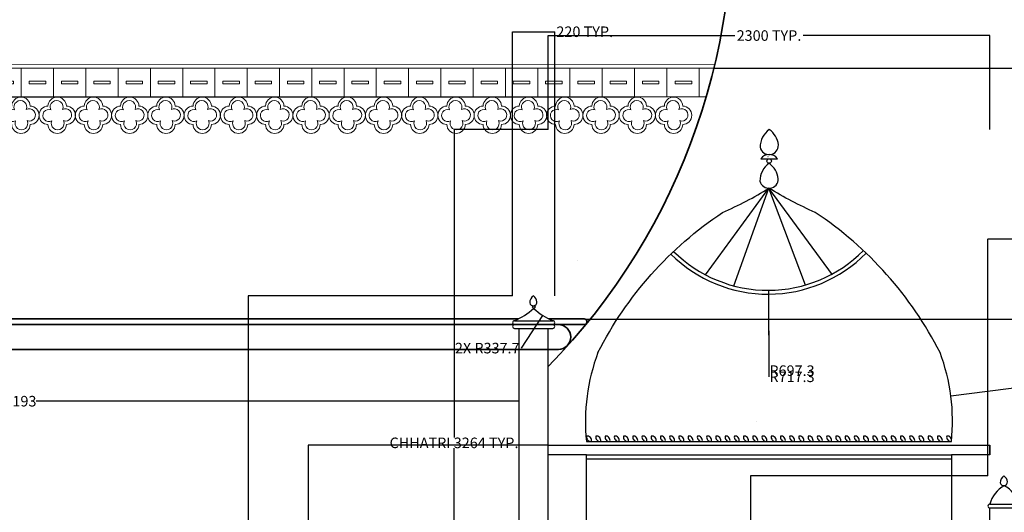
# Model space of a CAD drawing. Units: millimetres. Extents: x 8570 to 49085, y 3782 to 24863.
# Tile 7 of 15: x 22404 to 27529, y 15269 to 17835. Entities that reach past the tile are written whole.
import ezdxf

# ---------------------------------------------------------------- set-up
doc = ezdxf.new("R2010")
doc.units = ezdxf.units.MM
doc.header["$MEASUREMENT"] = 0
doc.header["$PDMODE"] = 3
for name, color, linetype, lineweight in [('A-ANNO-DIMS', 2, 'Continuous', 18), ('A-ELEV-ORNM', 7, 'Continuous', 13), ('A-ELEV-PIER', 7, 'Continuous', 25), ('A-ROOF-CHAT', 7, 'Continuous', 25), ('A-ROOF-DOME', 7, 'Continuous', 35)]:
    doc.layers.add(name, color=color, linetype=linetype, lineweight=lineweight)
doc.styles.get("Standard").update_dxf_attribs({"font": 'arial.ttf'})
doc.dimstyles.get("Standard").update_dxf_attribs({"dimtxt": 55, "dimasz": 0.18, "dimexe": 0.18, "dimexo": 0.0625, "dimgap": 0.09, "dimtad": 0, "dimtih": 1, "dimtoh": 1, "dimdec": 0, "dimzin": 0, "dimdsep": 46, "dimtxsty": 'Standard', "dimcen": 0.09, "dimadec": 0, "dimazin": 0, "dimtfac": 1, "dimtdec": 0, "dimtofl": 0, "dimtmove": 0, "dimatfit": 3, "dimfxl": 1, "dimtolj": 1, "dimtzin": 0, "dimarcsym": 0})

# ---------------------------------------------------------------- blocks, each defined once
blk = doc.blocks.new('DOME-QUATREFOIL')
for points in [[(46.6, 142.6, -0.970905), (142.6, 142.6, -0.014762)], [(60.6, 123.5, -1.525971), (122.6, 123.9, -0.970905)], [(46.6, 142.6, 0.970905), (46.6, 46.6, 0.014762)], [(63.1, 122.6, 1.61118), (66.6, 66.4, 0.970905)], [(122.6, 123.9, -1.560941), (127.1, 66.6, -0.970905)], [(142.6, 142.6, -0.970905), (142.6, 46.6, -0.014762)], [(66.6, 66.4, 1.55908), (127.1, 66.6, 0.970905)], [(46.6, 46.6, 0.970905), (142.6, 46.6, 0.014762)]]:
    blk.add_lwpolyline(points, format="xyb")
blk = doc.blocks.new('DOME-FRIEZE-PANEL')
for points in [[(0, 150), (168, 150), (168, 0), (0, 0)], [(41, 82), (127, 82), (127, 68), (41, 68)]]:
    blk.add_lwpolyline(points, close=True)
blk = doc.blocks.new('IWAN-EDGE-PINNACLE')
for p, q in [((10, 9044.5), (210, 9044.5)), ((10, 9004.5), (210, 9004.5)), ((35, 0), (35, 9004.5)), ((185, 0), (185, 9004.5))]:
    blk.add_line(p, q)
blk.add_lwpolyline([(127.1, 9142.4, 0.216309), (108.4, 9173.9, 0.244698), (89.5, 9137.5, 0.244698)], format="xyb")
blk.add_circle((110.5, 9116), 7.02)
for centre, radius, start, end in [((108.1, 9141.9), 19, 193.3065, 1.388), ((-119.7, 9355.4), 336.9, 292.6494, 312.9946), ((340.2, 9356.1), 337.7, 227.0303, 247.3257), ((10, 9034.5), 10, 90, 270), ((10, 9014.5), 10, 90, 270), ((210, 9034.5), 10, 270, 90), ((210, 9014.5), 10, 270, 90)]:
    blk.add_arc(centre, radius, start, end)
blk = doc.blocks.new('PAVILION-EDGE-PINNACLE')
for p, q in [((10, 8089.5), (160, 8089.5)), ((10, 0), (10, 8069.5)), ((10, 8069.5), (160, 8069.5))]:
    blk.add_line(p, q)
blk.add_lwpolyline([(101.6, 8204.8, 0.216309), (82.9, 8236.3, 0.244698), (64, 8200, 0.244698)], format="xyb")
for centre, radius, start, end in [((82.6, 8204.4), 19, 193.3065, 1.388), ((153, 8055.1), 147, 117.5278, 166.4748), ((17, 8055.1), 147, 13.5252, 62.4722), ((10, 8079.5), 10, 90, 270)]:
    blk.add_arc(centre, radius, start, end)
blk = doc.blocks.new('CHHATRI-ELEV')
for p, q in [((1107.1, 3111.9), (1194.6, 3111.9)), ((819.3, 2507.3), (1150, 2958.1)), ((967.4, 2449.5), (1150, 2958.1)), ((1480.7, 2507.3), (1150, 2958.1)), ((1339.8, 2454.2), (1150, 2958.1)), ((200, 1639.5), (2100, 1639.5)), ((2300, 1569.5), (2300, 1619.5)), ((200, 1549.5), (2100, 1549.5)), ((610, 0), (610, 754)), ((800, 0), (800, 754)), ((1500, 0), (1500, 744.5)), ((1692, 0), (1692, 744.5)), ((610, 158.5), (200, 158.5)), ((800, 158.5), (1500, 158.5)), ((2100, 158.5), (1692, 158.5))]:
    blk.add_line(p, q)
for points in [[(1199.3, 3183.7, 0.216309), (1151.6, 3264, 0.244698), (1103.6, 3171.4, 0.244698)], [(1198.5, 3007.8, 0.216309), (1150.8, 3088.1, 0.244698), (1102.8, 2995.4, 0.244698)], [(259.6, 2102.5, -0.128405), (908.9, 2832.4, 0.03556), (1150, 2958.1)], [(2040.4, 2102.5, 0.128405), (1391.1, 2832.4, -0.03556), (1150, 2958.1)]]:
    blk.add_lwpolyline(points, format="xyb")
for points in [[(225.8, 1639.5, 0.520567), (200.9, 1667.5, 0.520567)], [(273.9, 1639.5, 0.520567), (249, 1667.5, 0.520567)], [(321.9, 1639.5, 0.520567), (297.1, 1667.5, 0.520567)], [(370, 1639.5, 0.520567), (345.1, 1667.5, 0.520567)], [(418, 1639.5, 0.520567), (393.2, 1667.5, 0.520567)], [(466.1, 1639.5, 0.520567), (441.2, 1667.5, 0.520567)], [(514.2, 1639.5, 0.520567), (489.3, 1667.5, 0.520567)], [(562.2, 1639.5, 0.520567), (537.3, 1667.5, 0.520567)], [(610.3, 1639.5, 0.520567), (585.4, 1667.5, 0.520567)], [(658.3, 1639.5, 0.520567), (633.4, 1667.5, 0.520567)], [(706.4, 1639.5, 0.520567), (681.5, 1667.5, 0.520567)], [(754.4, 1639.5, 0.520567), (729.6, 1667.5, 0.520567)], [(802.5, 1639.5, 0.520567), (777.6, 1667.5, 0.520567)], [(850.5, 1639.5, 0.520567), (825.7, 1667.5, 0.520567)], [(898.6, 1639.5, 0.520567), (873.7, 1667.5, 0.520567)], [(946.7, 1639.5, 0.520567), (921.8, 1667.5, 0.520567)], [(994.7, 1639.5, 0.520567), (969.8, 1667.5, 0.520567)], [(1042.8, 1639.5, 0.520567), (1017.9, 1667.5, 0.520567)], [(1090.8, 1639.5, 0.520567), (1065.9, 1667.5, 0.520567)], [(1138.9, 1639.5, 0.520567), (1114, 1667.5, 0.520567)], [(1186.9, 1639.5, 0.520567), (1162.1, 1667.5, 0.520567)], [(1235, 1639.5, 0.520567), (1210.1, 1667.5, 0.520567)], [(1283, 1639.5, 0.520567), (1258.2, 1667.5, 0.520567)], [(1331.1, 1639.5, 0.520567), (1306.2, 1667.5, 0.520567)], [(1379.2, 1639.5, 0.520567), (1354.3, 1667.5, 0.520567)], [(1427.2, 1639.5, 0.520567), (1402.3, 1667.5, 0.520567)], [(1475.3, 1639.5, 0.520567), (1450.4, 1667.5, 0.520567)], [(1523.3, 1639.5, 0.520567), (1498.4, 1667.5, 0.520567)], [(1571.4, 1639.5, 0.520567), (1546.5, 1667.5, 0.520567)], [(1619.4, 1639.5, 0.520567), (1594.6, 1667.5, 0.520567)], [(1667.5, 1639.5, 0.520567), (1642.6, 1667.5, 0.520567)], [(1715.6, 1639.5, 0.520567), (1690.7, 1667.5, 0.520567)], [(1763.6, 1639.5, 0.520567), (1738.7, 1667.5, 0.520567)], [(1811.7, 1639.5, 0.520567), (1786.8, 1667.5, 0.520567)], [(1859.7, 1639.5, 0.520567), (1834.8, 1667.5, 0.520567)], [(1907.8, 1639.5, 0.520567), (1882.9, 1667.5, 0.520567)], [(1955.8, 1639.5, 0.520567), (1931, 1667.5, 0.520567)], [(2003.9, 1639.5, 0.520567), (1979, 1667.5, 0.520567)], [(2051.9, 1639.5, 0.520567), (2027.1, 1667.5, 0.520567)], [(2100, 1639.5, 0.520567), (2075.1, 1667.5, 0.520567)]]:
    blk.add_lwpolyline(points, format="xyb", close=True)
for points in [[(200, 1569.5), (0, 1569.5), (0, 1619.5), (2300, 1619.5), (2300, 1569.5), (2100, 1569.5)], [(2100, 0), (200, 0), (200, 1569.5), (2100, 1569.5), (2100, 0)]]:
    blk.add_lwpolyline(points)
blk.add_circle((1150.8, 3100), 11.9)
for centre, radius, start, end in [((1150.8, 3182.5), 48.5, 193.3065, 1.388), ((1150.8, 3079.7), 54.3, 36.3748, 143.6252), ((1150, 3006.6), 48.5, 193.3065, 1.388), ((1145, 3123.8), 717.3, 225.1557, 315.3968), ((1145, 3123.8), 697.3, 225.1557, 315.3968), ((1217.2, 1743.8), 1022.5, 159.4655, 185.8543), ((1082.8, 1743.8), 1022.5, 354.1457, 20.5345), ((260.1, 742.6), 350.1, 358.1332, 99.8832), ((1149.9, 742.6), 350.1, 359.6883, 181.8668), ((2042.1, 742.6), 350.1, 80.4789, 180.3117)]:
    blk.add_arc(centre, radius, start, end)
blk = doc.blocks.new('*D19')
at = {"layer": 'A-ANNO-DIMS', "color": 0, "lineweight": -2, "transparency": 16777216}
for p, q in [((24968.9, 16396.4), (23592.7, 16396.4)), ((23592.9, 16396.2), (23592.9, 11838)), ((23592.9, 7222.7), (23592.9, 11780.9)), ((24968.9, 7222.5), (23592.7, 7222.5))]:
    blk.add_line(p, q, dxfattribs=at)
at = {"layer": 'A-ANNO-DIMS', "color": 0, "transparency": 16777216}
for points in [[(23592.9, 16396.2), (23593, 16396.2), (23592.9, 16396.4)], [(23592.9, 7222.7), (23593, 7222.7), (23592.9, 7222.5)]]:
    blk.add_solid(points, dxfattribs=at)
at = {"layer": 'Defpoints', "color": 0, "transparency": 16777216}
for p in [(23592.9, 16396.4), (24969, 16396.4), (24969, 7222.5)]:
    blk.add_point(p, dxfattribs=at)
at = {"layer": 'A-ANNO-DIMS', "color": 0, "transparency": 16777216, "insert": (23592.9, 11809.4), "char_height": 55, "attachment_point": 5}
blk.add_mtext('\\A1;IWAN PINNACLE 9174 TYP.', dxfattribs=at)
blk = doc.blocks.new('*D20')
at = {"layer": 'A-ANNO-DIMS', "color": 0, "lineweight": -2, "transparency": 16777216}
for p, q in [((24969, 16396.4), (24969, 17772.6)), ((24969.2, 17772.4), (25188.8, 17772.4)), ((25189, 16396.4), (25189, 17772.6)), ((25189, 17772.4), (25189.2, 17772.4))]:
    blk.add_line(p, q, dxfattribs=at)
at = {"layer": 'A-ANNO-DIMS', "color": 0, "transparency": 16777216}
for points in [[(24969.2, 17772.5), (24969.2, 17772.4), (24969, 17772.4)], [(25188.8, 17772.5), (25188.8, 17772.4), (25189, 17772.4)]]:
    blk.add_solid(points, dxfattribs=at)
at = {"layer": 'Defpoints', "color": 0, "transparency": 16777216}
for p in [(25189, 17772.4), (24969, 16396.4), (25189, 16396.4)]:
    blk.add_point(p, dxfattribs=at)
at = {"layer": 'A-ANNO-DIMS', "color": 0, "transparency": 16777216, "insert": (25345, 17772.4), "char_height": 55, "attachment_point": 5}
blk.add_mtext('\\A1;220 TYP.', dxfattribs=at)
blk = doc.blocks.new('*D21')
at = {"layer": 'A-ANNO-DIMS', "color": 0, "lineweight": -2, "transparency": 16777216}
for p, q in [((27443.9, 15458.8), (26208.4, 15458.8)), ((26208.5, 15458.7), (26208.5, 11369.2)), ((26208.5, 7222.7), (26208.5, 11312.1)), ((27443.9, 7222.5), (26208.4, 7222.5))]:
    blk.add_line(p, q, dxfattribs=at)
at = {"layer": 'A-ANNO-DIMS', "color": 0, "transparency": 16777216}
for points in [[(26208.5, 15458.7), (26208.6, 15458.7), (26208.5, 15458.8)], [(26208.5, 7222.7), (26208.6, 7222.7), (26208.5, 7222.5)]]:
    blk.add_solid(points, dxfattribs=at)
at = {"layer": 'Defpoints', "color": 0, "transparency": 16777216}
for p in [(26208.5, 15458.8), (27444, 15458.8), (27444, 7222.5)]:
    blk.add_point(p, dxfattribs=at)
at = {"layer": 'A-ANNO-DIMS', "color": 0, "transparency": 16777216, "insert": (26208.5, 11340.7), "char_height": 55, "attachment_point": 5}
blk.add_mtext('\\A1;PAVILION PINNACLE 8236 TYP.', dxfattribs=at)
blk = doc.blocks.new('*D22')
at = {"layer": 'A-ANNO-DIMS', "color": 0, "lineweight": -2, "transparency": 16777216}
for p, q in [((27444, 15458.9), (27444, 16694.5)), ((27444.2, 16694.3), (27613.8, 16694.3)), ((27614, 15458.9), (27614, 16694.5)), ((27614, 16694.3), (27614.2, 16694.3))]:
    blk.add_line(p, q, dxfattribs=at)
at = {"layer": 'A-ANNO-DIMS', "color": 0, "transparency": 16777216}
for points in [[(27444.2, 16694.3), (27444.2, 16694.3), (27444, 16694.3)], [(27613.8, 16694.3), (27613.8, 16694.3), (27614, 16694.3)]]:
    blk.add_solid(points, dxfattribs=at)
at = {"layer": 'Defpoints', "color": 0, "transparency": 16777216}
for p in [(27614, 16694.3), (27444, 15458.8), (27614, 15458.8)]:
    blk.add_point(p, dxfattribs=at)
at = {"layer": 'A-ANNO-DIMS', "color": 0, "transparency": 16777216, "insert": (27766.9, 16694.3), "char_height": 55, "attachment_point": 5}
blk.add_mtext('\\A1;170 TYP.', dxfattribs=at)
blk = doc.blocks.new('*D25')
at = {"layer": 'A-ANNO-DIMS', "color": 0, "lineweight": -2, "transparency": 16777216}
for p, q in [((25153.9, 17263), (24664.2, 17263)), ((24664.4, 17262.9), (24664.4, 15659.6)), ((24664.4, 13999.2), (24664.4, 15602.5)), ((25153.9, 13999), (24664.2, 13999))]:
    blk.add_line(p, q, dxfattribs=at)
at = {"layer": 'A-ANNO-DIMS', "color": 0, "transparency": 16777216}
for points in [[(24664.4, 17262.9), (24664.4, 17262.9), (24664.4, 17263)], [(24664.4, 13999.2), (24664.4, 13999.2), (24664.4, 13999)]]:
    blk.add_solid(points, dxfattribs=at)
at = {"layer": 'Defpoints', "color": 0, "transparency": 16777216}
for p in [(24664.4, 17263), (25154, 17263), (25154, 13999)]:
    blk.add_point(p, dxfattribs=at)
at = {"layer": 'A-ANNO-DIMS', "color": 0, "transparency": 16777216, "insert": (24664.4, 15631), "char_height": 55, "attachment_point": 5}
blk.add_mtext('\\A1;CHHATRI 3264 TYP.', dxfattribs=at)
blk = doc.blocks.new('*D26')
at = {"layer": 'A-ANNO-DIMS', "color": 0, "lineweight": -2, "transparency": 16777216}
for p, q in [((25154, 17263.1), (25154, 17752.8)), ((25154.2, 17752.6), (26126.8, 17752.6)), ((27453.8, 17752.6), (26481.2, 17752.6)), ((27454, 17263.1), (27454, 17752.8))]:
    blk.add_line(p, q, dxfattribs=at)
at = {"layer": 'A-ANNO-DIMS', "color": 0, "transparency": 16777216}
for points in [[(25154.2, 17752.7), (25154.2, 17752.6), (25154, 17752.6)], [(27453.8, 17752.7), (27453.8, 17752.6), (27454, 17752.6)]]:
    blk.add_solid(points, dxfattribs=at)
at = {"layer": 'Defpoints', "color": 0, "transparency": 16777216}
for p in [(27454, 17752.6), (25154, 17263), (27454, 17263)]:
    blk.add_point(p, dxfattribs=at)
at = {"layer": 'A-ANNO-DIMS', "color": 0, "transparency": 16777216, "insert": (26304, 17752.6), "char_height": 55, "attachment_point": 5}
blk.add_mtext('\\A1;2300 TYP.', dxfattribs=at)
blk = doc.blocks.new('*D47')
at = {"layer": 'A-ANNO-DIMS', "color": 0, "lineweight": -2, "transparency": 16777216}
for p, q in [((19811, 14600.1), (19811, 15848.2)), ((19811.2, 15848), (22325.3, 15848)), ((25003.8, 15848), (22489.7, 15848)), ((25004, 14600.1), (25004, 15848.2))]:
    blk.add_line(p, q, dxfattribs=at)
at = {"layer": 'A-ANNO-DIMS', "color": 0, "transparency": 16777216}
for points in [[(19811.2, 15848), (19811.2, 15848), (19811, 15848)], [(25003.8, 15848), (25003.8, 15848), (25004, 15848)]]:
    blk.add_solid(points, dxfattribs=at)
at = {"layer": 'Defpoints', "color": 0, "transparency": 16777216}
for p in [(25004, 15848), (19811, 14600), (25004, 14600)]:
    blk.add_point(p, dxfattribs=at)
at = {"layer": 'A-ANNO-DIMS', "color": 0, "transparency": 16777216, "insert": (22407.5, 15848), "char_height": 55, "attachment_point": 5}
blk.add_mtext('\\A1;5193', dxfattribs=at)
blk = doc.blocks.new('*D53')
at = {"layer": 'A-ANNO-DIMS', "color": 0, "lineweight": -2, "transparency": 16777216}
for p, q in [((26017.6, 17582.8), (36055.2, 17582.8)), ((36055, 17582.6), (36055, 16957.5)), ((36055, 16276), (36055, 16901.1)), ((25347.4, 16275.8), (36055.2, 16275.8))]:
    blk.add_line(p, q, dxfattribs=at)
at = {"layer": 'A-ANNO-DIMS', "color": 0, "transparency": 16777216}
for points in [[(36055, 17582.6), (36055, 17582.6), (36055, 17582.8)], [(36055, 16276), (36055, 16276), (36055, 16275.8)]]:
    blk.add_solid(points, dxfattribs=at)
at = {"layer": 'Defpoints', "color": 0, "transparency": 16777216}
for p in [(26017.6, 17582.8), (36055, 17582.8), (25347.3, 16275.8)]:
    blk.add_point(p, dxfattribs=at)
at = {"layer": 'A-ANNO-DIMS', "color": 0, "transparency": 16777216, "insert": (36055, 16929.3), "char_height": 55, "attachment_point": 5}
blk.add_mtext('\\A1;1307', dxfattribs=at)
blk = doc.blocks.new('*D54')
at = {"layer": 'A-ANNO-DIMS', "color": 0, "lineweight": -2, "transparency": 16777216}
for p, q in [((24765.7, 21387.4), (36055.2, 21387.4)), ((36055, 21387.2), (36055, 19513.3)), ((36055, 17583), (36055, 19456.9)), ((26017.6, 17582.8), (36055.2, 17582.8))]:
    blk.add_line(p, q, dxfattribs=at)
at = {"layer": 'A-ANNO-DIMS', "color": 0, "transparency": 16777216}
for points in [[(36055, 21387.2), (36055, 21387.2), (36055, 21387.4)], [(36055, 17583), (36055, 17583), (36055, 17582.8)]]:
    blk.add_solid(points, dxfattribs=at)
at = {"layer": 'Defpoints', "color": 0, "transparency": 16777216}
for p in [(24765.6, 21387.4), (36055, 21387.4), (26017.6, 17582.8)]:
    blk.add_point(p, dxfattribs=at)
at = {"layer": 'A-ANNO-DIMS', "color": 0, "transparency": 16777216, "insert": (36055, 19485.1), "char_height": 55, "attachment_point": 5}
blk.add_mtext('\\A1;3804.6', dxfattribs=at)
blk = doc.blocks.new('*D61')
at = {"layer": 'A-ANNO-DIMS', "color": 0, "lineweight": -2, "transparency": 16777216}
for p, q in [((33091.4, 17974), (8684.3, 17974)), ((8684.5, 17973.8), (8684.5, 15935.4)), ((8684.5, 13840.7), (8684.5, 15879.1)), ((33041.4, 13840.5), (8684.3, 13840.5))]:
    blk.add_line(p, q, dxfattribs=at)
at = {"layer": 'A-ANNO-DIMS', "color": 0, "transparency": 16777216}
for points in [[(8684.5, 17973.8), (8684.5, 17973.8), (8684.5, 17974)], [(8684.5, 13840.7), (8684.5, 13840.7), (8684.5, 13840.5)]]:
    blk.add_solid(points, dxfattribs=at)
at = {"layer": 'Defpoints', "color": 0, "transparency": 16777216}
for p in [(8684.5, 17974), (33091.5, 17974), (33041.5, 13840.5)]:
    blk.add_point(p, dxfattribs=at)
at = {"layer": 'A-ANNO-DIMS', "color": 0, "transparency": 16777216, "insert": (8684.5, 15907.2), "char_height": 55, "attachment_point": 5}
blk.add_mtext('\\A1;4133.5', dxfattribs=at)
blk = doc.blocks.new('*D69')
at = {"layer": 'A-ANNO-DIMS', "color": 0, "lineweight": -2, "transparency": 16777216}
for p, q in [((25153.9, 15618.5), (23905.8, 15618.5)), ((23906, 15618.3), (23906, 14836.9)), ((23906, 13999.2), (23906, 14780.6)), ((25153.9, 13999), (23905.8, 13999))]:
    blk.add_line(p, q, dxfattribs=at)
at = {"layer": 'A-ANNO-DIMS', "color": 0, "transparency": 16777216}
for points in [[(23906, 15618.3), (23906, 15618.3), (23906, 15618.5)], [(23906, 13999.2), (23906, 13999.2), (23906, 13999)]]:
    blk.add_solid(points, dxfattribs=at)
at = {"layer": 'Defpoints', "color": 0, "transparency": 16777216}
for p in [(23906, 15618.5), (25154, 15618.5), (25154, 13999)]:
    blk.add_point(p, dxfattribs=at)
at = {"layer": 'A-ANNO-DIMS', "color": 0, "transparency": 16777216, "insert": (23906, 14808.7), "char_height": 55, "attachment_point": 5}
blk.add_mtext('\\A1;1619.5', dxfattribs=at)
blk = doc.blocks.new('*D87')
at = {"layer": 'A-ANNO-DIMS', "color": 0, "lineweight": -2, "transparency": 16777216}
for p, q in [((27859.4, 15951.8), (27251.1, 15873.5)), ((26236.7, 15742.8), (26236.9, 15742.8)), ((26236.8, 15742.7), (26236.8, 15742.9))]:
    blk.add_line(p, q, dxfattribs=at)
at = {"layer": 'A-ANNO-DIMS', "color": 0, "transparency": 16777216}
blk.add_solid([(27251.1, 15873.5), (27251.1, 15873.4), (27251, 15873.4)], dxfattribs=at)
at = {"layer": 'Defpoints', "color": 0, "transparency": 16777216}
for p in [(27251, 15873.4), (26236.8, 15742.8)]:
    blk.add_point(p, dxfattribs=at)
at = {"layer": 'A-ANNO-DIMS', "color": 0, "transparency": 16777216, "insert": (28059.8, 15951.8), "char_height": 55, "attachment_point": 5}
blk.add_mtext('\\A1;2X R1022.5', dxfattribs=at)
blk = doc.blocks.new('*D89')
at = {"layer": 'A-ANNO-DIMS', "color": 0, "lineweight": -2, "transparency": 16777216}
for p, q in [((26298.9, 17122.8), (26299.1, 17122.8)), ((26299, 17122.7), (26299, 17122.8)), ((26304.5, 15975.1), (26302.5, 16405.3)), ((26304.7, 15975.1), (26304.5, 15975.1))]:
    blk.add_line(p, q, dxfattribs=at)
at = {"layer": 'A-ANNO-DIMS', "color": 0, "transparency": 16777216}
blk.add_solid([(26302.5, 16405.3), (26302.4, 16405.3), (26302.5, 16405.5)], dxfattribs=at)
at = {"layer": 'Defpoints', "color": 0, "transparency": 16777216}
for p in [(26299, 17122.8), (26302.5, 16405.5)]:
    blk.add_point(p, dxfattribs=at)
at = {"layer": 'A-ANNO-DIMS', "color": 0, "transparency": 16777216, "insert": (26423.9, 15975.1), "char_height": 55, "attachment_point": 5}
blk.add_mtext('\\A1;R717.3', dxfattribs=at)
blk = doc.blocks.new('*D90')
at = {"layer": 'A-ANNO-DIMS', "color": 0, "lineweight": -2, "transparency": 16777216}
for p, q in [((26298.9, 17122.8), (26299.1, 17122.8)), ((26299, 17122.7), (26299, 17122.8)), ((26304.4, 16007.1), (26302.4, 16425.3)), ((26304.6, 16007.1), (26304.4, 16007.1))]:
    blk.add_line(p, q, dxfattribs=at)
at = {"layer": 'A-ANNO-DIMS', "color": 0, "transparency": 16777216}
blk.add_solid([(26302.4, 16425.3), (26302.3, 16425.3), (26302.4, 16425.5)], dxfattribs=at)
at = {"layer": 'Defpoints', "color": 0, "transparency": 16777216}
for p in [(26299, 17122.8), (26302.4, 16425.5)]:
    blk.add_point(p, dxfattribs=at)
at = {"layer": 'A-ANNO-DIMS', "color": 0, "transparency": 16777216, "insert": (26423.8, 16007.1), "char_height": 55, "attachment_point": 5}
blk.add_mtext('\\A1;R697.3', dxfattribs=at)
blk = doc.blocks.new('*D92')
at = {"layer": 'A-ANNO-DIMS', "color": 0, "lineweight": -2, "transparency": 16777216}
for p, q in [((25309.1, 16578.6), (25309.3, 16578.6)), ((25309.2, 16578.5), (25309.2, 16578.7)), ((25016.3, 16124.5), (25126, 16294.7)), ((25016.1, 16124.5), (25016.3, 16124.5))]:
    blk.add_line(p, q, dxfattribs=at)
at = {"layer": 'A-ANNO-DIMS', "color": 0, "transparency": 16777216}
blk.add_solid([(25126, 16294.7), (25126.1, 16294.6), (25126.1, 16294.8)], dxfattribs=at)
at = {"layer": 'Defpoints', "color": 0, "transparency": 16777216}
for p in [(25309.2, 16578.6), (25126.1, 16294.8)]:
    blk.add_point(p, dxfattribs=at)
at = {"layer": 'A-ANNO-DIMS', "color": 0, "transparency": 16777216, "insert": (24837.4, 16124.5), "char_height": 55, "attachment_point": 5}
blk.add_mtext('\\A1;2X R337.7', dxfattribs=at)

msp = doc.modelspace()

# ---------------------------------------------------------------- linework, layer by layer
at = {"layer": 'A-ELEV-ORNM'}
for p, q in [((18793.79, 17602.41), (26022.36, 17602.82)), ((18798.6, 17582.41), (26017.56, 17582.82)), ((18838.91, 17432.42), (25940.01, 17432.81))]:
    msp.add_line(p, q, dxfattribs=at)
msp.add_lwpolyline([(25977.33, 17432.8), (25772.01, 17432.8), (25772.01, 17582.79), (25940.01, 17582.79), (25940.01, 17432.8)], dxfattribs=at)
msp.add_lwpolyline([(25816, 17514.42), (25902, 17514.42), (25902, 17500.42), (25816, 17500.42)], close=True, dxfattribs=at)
at = {"layer": 'A-ROOF-DOME'}
for p, q in [((19814.24, 16277), (25000.76, 16277)), ((25157.26, 16277), (25341.5, 16277)), ((19473.5, 16247), (25341.5, 16247)), ((19617, 16118), (25207.5, 16118))]:
    msp.add_line(p, q, dxfattribs=at)
for centre, radius, start, end in [((22756.66, 18376.72), 3356.15, 315.58696, 56.67466), ((25341.5, 16262), 15, 270, 90), ((25207.5, 16182.5), 64.5, 270, 90)]:
    msp.add_arc(centre, radius, start, end, dxfattribs=at)

# ---------------------------------------------------------------- block references
at = {"layer": 'A-ELEV-ORNM'}
for name, p in [('DOME-FRIEZE-PANEL', (22244.01, 17432.43)), ('DOME-FRIEZE-PANEL', (22412.01, 17432.43)), ('DOME-FRIEZE-PANEL', (22580.01, 17432.43)), ('DOME-FRIEZE-PANEL', (22748.01, 17432.43)), ('DOME-FRIEZE-PANEL', (22916.01, 17432.43)), ('DOME-FRIEZE-PANEL', (23084.01, 17432.43)), ('DOME-FRIEZE-PANEL', (23252.01, 17432.43)), ('DOME-FRIEZE-PANEL', (23420.01, 17432.43)), ('DOME-FRIEZE-PANEL', (23588.01, 17432.43)), ('DOME-FRIEZE-PANEL', (23756.01, 17432.43)), ('DOME-FRIEZE-PANEL', (23924.01, 17432.43)), ('DOME-FRIEZE-PANEL', (24092.01, 17432.43)), ('DOME-FRIEZE-PANEL', (24260.01, 17432.43)), ('DOME-FRIEZE-PANEL', (24428.01, 17432.43)), ('DOME-FRIEZE-PANEL', (24596.01, 17432.43)), ('DOME-FRIEZE-PANEL', (24764.01, 17432.43)), ('DOME-FRIEZE-PANEL', (24932.01, 17432.43)), ('DOME-FRIEZE-PANEL', (25100.01, 17432.43)), ('DOME-FRIEZE-PANEL', (25268.01, 17432.43)), ('DOME-FRIEZE-PANEL', (25436.01, 17432.43)), ('DOME-FRIEZE-PANEL', (25604.01, 17432.79)), ('DOME-QUATREFOIL', (22315.59, 17242.64)), ('DOME-QUATREFOIL', (22504.33, 17242.64)), ('DOME-QUATREFOIL', (22693.06, 17242.64)), ('DOME-QUATREFOIL', (22881.79, 17242.64)), ('DOME-QUATREFOIL', (23070.52, 17242.64)), ('DOME-QUATREFOIL', (23259.26, 17242.64)), ('DOME-QUATREFOIL', (23447.99, 17242.64)), ('DOME-QUATREFOIL', (23636.72, 17242.64)), ('DOME-QUATREFOIL', (23825.46, 17242.64)), ('DOME-QUATREFOIL', (24014.19, 17242.64)), ('DOME-QUATREFOIL', (24202.92, 17242.64)), ('DOME-QUATREFOIL', (24391.66, 17242.64)), ('DOME-QUATREFOIL', (24580.39, 17242.64)), ('DOME-QUATREFOIL', (24769.12, 17242.64)), ('DOME-QUATREFOIL', (24957.85, 17242.64)), ('DOME-QUATREFOIL', (25146.59, 17242.64)), ('DOME-QUATREFOIL', (25335.32, 17242.64)), ('DOME-QUATREFOIL', (25524.05, 17242.64)), ('DOME-QUATREFOIL', (25712.79, 17242.64))]:
    msp.add_blockref(name, p, dxfattribs=at)
at = {"layer": 'A-ELEV-PIER'}
for name, p in [('IWAN-EDGE-PINNACLE', (24969, 7222.5)), ('PAVILION-EDGE-PINNACLE', (27444, 7222.5))]:
    msp.add_blockref(name, p, dxfattribs=at)
at = {"layer": 'A-ROOF-CHAT'}
msp.add_blockref('CHHATRI-ELEV', (25154, 13999), dxfattribs=at)

# ---------------------------------------------------------------- dimensions: what is measured, and where the dimension line sits
at = {"layer": 'A-ANNO-DIMS'}
for base, p1, p2, override, picture, middle in [((36055, 21387.41), (26017.56, 17582.82), (24765.63, 21387.41), {"dimdec": 1, "dimlfac": 1, "dimrnd": 0, "dimzin": 0, "dimdsep": 46, "dimlunit": 2}, '*D54', (36055, 19485.11)), ((8684.5, 17974), (33041.5, 13840.5), (33091.5, 17974), {"dimdec": 1, "dimlfac": 1, "dimrnd": 0, "dimzin": 0, "dimdsep": 46, "dimlunit": 2}, '*D61', (8684.5, 15907.25)), ((36055, 17582.82), (25347.34, 16275.82), (26017.56, 17582.82), {"dimdec": 0, "dimlfac": 1, "dimrnd": 0, "dimzin": 0, "dimdsep": 46, "dimlunit": 2}, '*D53', (36055, 16929.32)), ((23906, 15618.5), (25154, 13999), (25154, 15618.5), {"dimdec": 1, "dimlfac": 1, "dimrnd": 0, "dimzin": 0, "dimdsep": 46, "dimlunit": 2}, '*D69', (23906, 14808.75))]:
    dim = msp.add_linear_dim(base=base, p1=p1, p2=p2, angle=90, dimstyle='Standard', override=override, dxfattribs=at)
    dim.commit()
    dim.dimension.update_dxf_attribs({"geometry": picture, "text_midpoint": middle})
for base, p1, p2, picture, middle in [((25189, 17772.44), (24969, 16396.36), (25189, 16396.36), '*D20', (25344.97, 17772.44)), ((27454, 17752.64), (25154, 17263.04), (27454, 17263.04), '*D26', (26304, 17752.64)), ((27614, 16694.3), (27444, 15458.84), (27614, 15458.84), '*D22', (27766.91, 16694.3))]:
    dim = msp.add_linear_dim(base=base, p1=p1, p2=p2, text='<> TYP.', dimstyle='Standard', override={"dimdec": 0, "dimlfac": 1, "dimrnd": 0, "dimzin": 0, "dimdsep": 46, "dimlunit": 2}, dxfattribs=at)
    dim.commit()
    dim.dimension.update_dxf_attribs({"geometry": picture, "text_midpoint": middle})
for base, p1, p2, text, picture, middle in [((24664.39, 17263.04), (25154, 13999), (25154, 17263.04), 'CHHATRI <> TYP.', '*D25', (24664.39, 15631.02)), ((23592.92, 16396.36), (24969, 7222.5), (24969, 16396.36), 'IWAN PINNACLE <> TYP.', '*D19', (23592.92, 11809.43)), ((26208.55, 15458.84), (27444, 7222.5), (27444, 15458.84), 'PAVILION PINNACLE <> TYP.', '*D21', (26208.55, 11340.67))]:
    dim = msp.add_linear_dim(base=base, p1=p1, p2=p2, angle=90, text=text, dimstyle='Standard', override={"dimdec": 0, "dimlfac": 1, "dimrnd": 0, "dimzin": 0, "dimdsep": 46, "dimlunit": 2}, dxfattribs=at)
    dim.commit()
    dim.dimension.update_dxf_attribs({"geometry": picture, "text_midpoint": middle})
for mpoint, picture, middle in [((26302.47, 16405.5), '*D89', (26423.93, 15975.14)), ((26302.37, 16425.5), '*D90', (26423.78, 16007.14))]:
    dim = msp.add_radius_dim(center=(26299.01, 17122.76), mpoint=mpoint, dimstyle='Standard', override={"dimdec": 1, "dimlfac": 1, "dimrnd": 0, "dimzin": 0, "dimdsep": 46, "dimlunit": 2}, dxfattribs=at)
    dim.commit()
    dim.dimension.update_dxf_attribs({"geometry": picture, "text_midpoint": middle, "dimtype": 164})
for center, mpoint, picture, middle in [((25309.18, 16578.6), (25126.14, 16294.81), '*D92', (24837.36, 16124.54)), ((26236.79, 15742.8), (27250.95, 15873.44), '*D87', (27859.45, 15951.82))]:
    dim = msp.add_radius_dim(center=center, mpoint=mpoint, text='2X <>', dimstyle='Standard', override={"dimdec": 1, "dimlfac": 1, "dimrnd": 0, "dimzin": 0, "dimdsep": 46, "dimlunit": 2}, dxfattribs=at)
    dim.commit()
    dim.dimension.update_dxf_attribs({"geometry": picture, "text_midpoint": middle, "dimtype": 164})
dim = msp.add_linear_dim(base=(25004, 15848), p1=(19811, 14600), p2=(25004, 14600), dimstyle='Standard', override={"dimdec": 0, "dimlfac": 1, "dimrnd": 0, "dimzin": 0, "dimdsep": 46, "dimlunit": 2}, dxfattribs=at)
dim.commit()
dim.dimension.update_dxf_attribs({"geometry": '*D47', "text_midpoint": (22407.5, 15848)})

doc.saveas('drawing.dxf')
